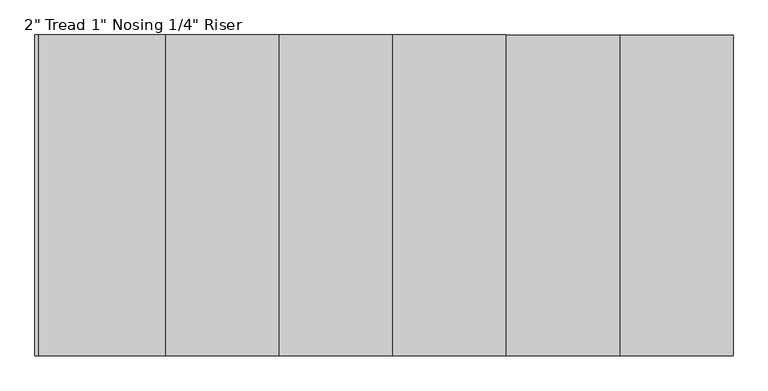
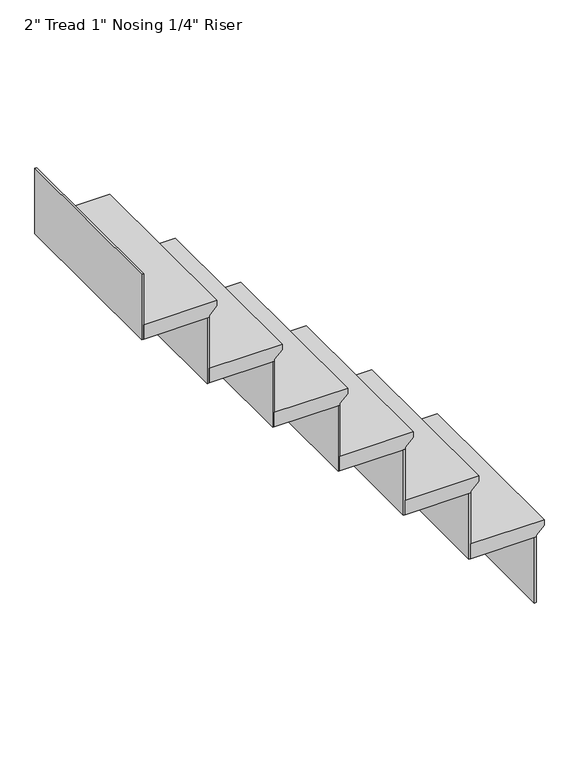
"""IFC4 building model written with IfcOpenShell, lengths in millimetres: stair flight geometry."""

from ifc_helpers import new_model, si_unit, frame, origin, place, context, project, spatial, polyline, outline, extrude, source, transform, mapped, element, save


def stair_flight_7576936b(model_context):
    return source(origin(), model_context, "Body", "SweptSolid", [
        extrude(outline(polyline([(5029.2, -3296.0237097), (5029.2, -3537.3237097), (4978.4, -3537.3237097), (4978.4, -3321.4237097), (4984.75, -3321.4237097), (5010.15, -3296.0237097), (5029.2, -3296.0237097)])), frame((0.0, 4341.1083475, 0.0), z_axis=(0.0, 1.0, 0.0), x_axis=(0.0, 0.0, 1.0)), (0.0, 0.0, 1.0), 609.6),
        extrude(outline(polyline([(-3327.7737097, 4950.7083475), (-3321.4237097, 4950.7083475), (-3321.4237097, 4341.1083475), (-3327.7737097, 4341.1083475), (-3327.7737097, 4950.7083475)])), frame((0.0, 0.0, 4749.8), z_axis=(0.0, 0.0, 1.0), x_axis=(1.0, 0.0, 0.0)), (0.0, 0.0, 1.0), 228.6),
        extrude(outline(polyline([(-4623.1737097, 4950.7083475), (-4616.8237097, 4950.7083475), (-4616.8237097, 4341.1083475), (-4623.1737097, 4341.1083475), (-4623.1737097, 4950.7083475)])), frame((0.0, 0.0, 6121.4), z_axis=(0.0, 0.0, 1.0), x_axis=(1.0, 0.0, 0.0)), (0.0, 0.0, 1.0), 228.6),
        extrude(outline(polyline([(-3543.6737097, 4950.7083475), (-3537.3237097, 4950.7083475), (-3537.3237097, 4341.1083475), (-3543.6737097, 4341.1083475), (-3543.6737097, 4950.7083475)])), frame((0.0, 0.0, 4978.4), z_axis=(0.0, 0.0, 1.0), x_axis=(1.0, 0.0, 0.0)), (0.0, 0.0, 1.0), 228.6),
        extrude(outline(polyline([(5257.8, -3511.9237097), (5257.8, -3753.2237097), (5207.0, -3753.2237097), (5207.0, -3537.3237097), (5213.35, -3537.3237097), (5238.75, -3511.9237097), (5257.8, -3511.9237097)])), frame((0.0, 4341.1083475, 0.0), z_axis=(0.0, 1.0, 0.0), x_axis=(0.0, 0.0, 1.0)), (0.0, 0.0, 1.0), 609.6),
        extrude(outline(polyline([(-3759.5737097, 4950.7083475), (-3753.2237097, 4950.7083475), (-3753.2237097, 4341.1083475), (-3759.5737097, 4341.1083475), (-3759.5737097, 4950.7083475)])), frame((0.0, 0.0, 5207.0), z_axis=(0.0, 0.0, 1.0), x_axis=(1.0, 0.0, 0.0)), (0.0, 0.0, 1.0), 228.6),
        extrude(outline(polyline([(5486.4, -3727.8237097), (5486.4, -3969.1237097), (5435.6, -3969.1237097), (5435.6, -3753.2237097), (5441.95, -3753.2237097), (5467.35, -3727.8237097), (5486.4, -3727.8237097)])), frame((0.0, 4341.1083475, 0.0), z_axis=(0.0, 1.0, 0.0), x_axis=(0.0, 0.0, 1.0)), (0.0, 0.0, 1.0), 609.6),
        extrude(outline(polyline([(-3975.4737097, 4950.7083475), (-3969.1237097, 4950.7083475), (-3969.1237097, 4341.1083475), (-3975.4737097, 4341.1083475), (-3975.4737097, 4950.7083475)])), frame((0.0, 0.0, 5435.6), z_axis=(0.0, 0.0, 1.0), x_axis=(1.0, 0.0, 0.0)), (0.0, 0.0, 1.0), 228.6),
        extrude(outline(polyline([(5715.0, -3943.7237097), (5715.0, -4185.0237097), (5664.2, -4185.0237097), (5664.2, -3969.1237097), (5670.55, -3969.1237097), (5695.95, -3943.7237097), (5715.0, -3943.7237097)])), frame((0.0, 4341.1083475, 0.0), z_axis=(0.0, 1.0, 0.0), x_axis=(0.0, 0.0, 1.0)), (0.0, 0.0, 1.0), 609.6),
        extrude(outline(polyline([(-4191.3737097, 4950.7083475), (-4185.0237097, 4950.7083475), (-4185.0237097, 4341.1083475), (-4191.3737097, 4341.1083475), (-4191.3737097, 4950.7083475)])), frame((0.0, 0.0, 5664.2), z_axis=(0.0, 0.0, 1.0), x_axis=(1.0, 0.0, 0.0)), (0.0, 0.0, 1.0), 228.6),
        extrude(outline(polyline([(5943.6, -4159.6237097), (5943.6, -4400.9237097), (5892.8, -4400.9237097), (5892.8, -4185.0237097), (5899.15, -4185.0237097), (5924.55, -4159.6237097), (5943.6, -4159.6237097)])), frame((0.0, 4341.1083475, 0.0), z_axis=(0.0, 1.0, 0.0), x_axis=(0.0, 0.0, 1.0)), (0.0, 0.0, 1.0), 609.6),
        extrude(outline(polyline([(-4407.2737097, 4950.7083475), (-4400.9237097, 4950.7083475), (-4400.9237097, 4341.1083475), (-4407.2737097, 4341.1083475), (-4407.2737097, 4950.7083475)])), frame((0.0, 0.0, 5892.8), z_axis=(0.0, 0.0, 1.0), x_axis=(1.0, 0.0, 0.0)), (0.0, 0.0, 1.0), 228.6),
        extrude(outline(polyline([(6172.2, -4375.5237097), (6172.2, -4616.8237097), (6121.4, -4616.8237097), (6121.4, -4400.9237097), (6127.75, -4400.9237097), (6153.15, -4375.5237097), (6172.2, -4375.5237097)])), frame((0.0, 4341.1083475, 0.0), z_axis=(0.0, 1.0, 0.0), x_axis=(0.0, 0.0, 1.0)), (0.0, 0.0, 1.0), 609.6),
    ])


if __name__ == "__main__":
    model = new_model("IFC4")
    model_context = context("Model", 3, world=origin())
    ifc_project = project(units=[si_unit("LENGTHUNIT", "METRE", prefix="MILLI")], contexts=[model_context])
    site = spatial("IfcSite", under=ifc_project)
    building = spatial("IfcBuilding", under=site)
    placement = place(None, origin())
    stair_flight_shape = stair_flight_7576936b(model_context)
    element("IfcStairFlight", 1, ObjectType="2\" Tread 1\" Nosing 1/4\" Riser", at=placement, inside=building, context=model_context, shape_type="MappedRepresentation", body=[
        mapped(stair_flight_shape, transform((0.0, 0.0, 0.0), x_axis=(1.0, 0.0, 0.0), y_axis=(0.0, 1.0, 0.0), z_axis=(0.0, 0.0, 1.0))),
    ])
    save(model, "model.ifc")
